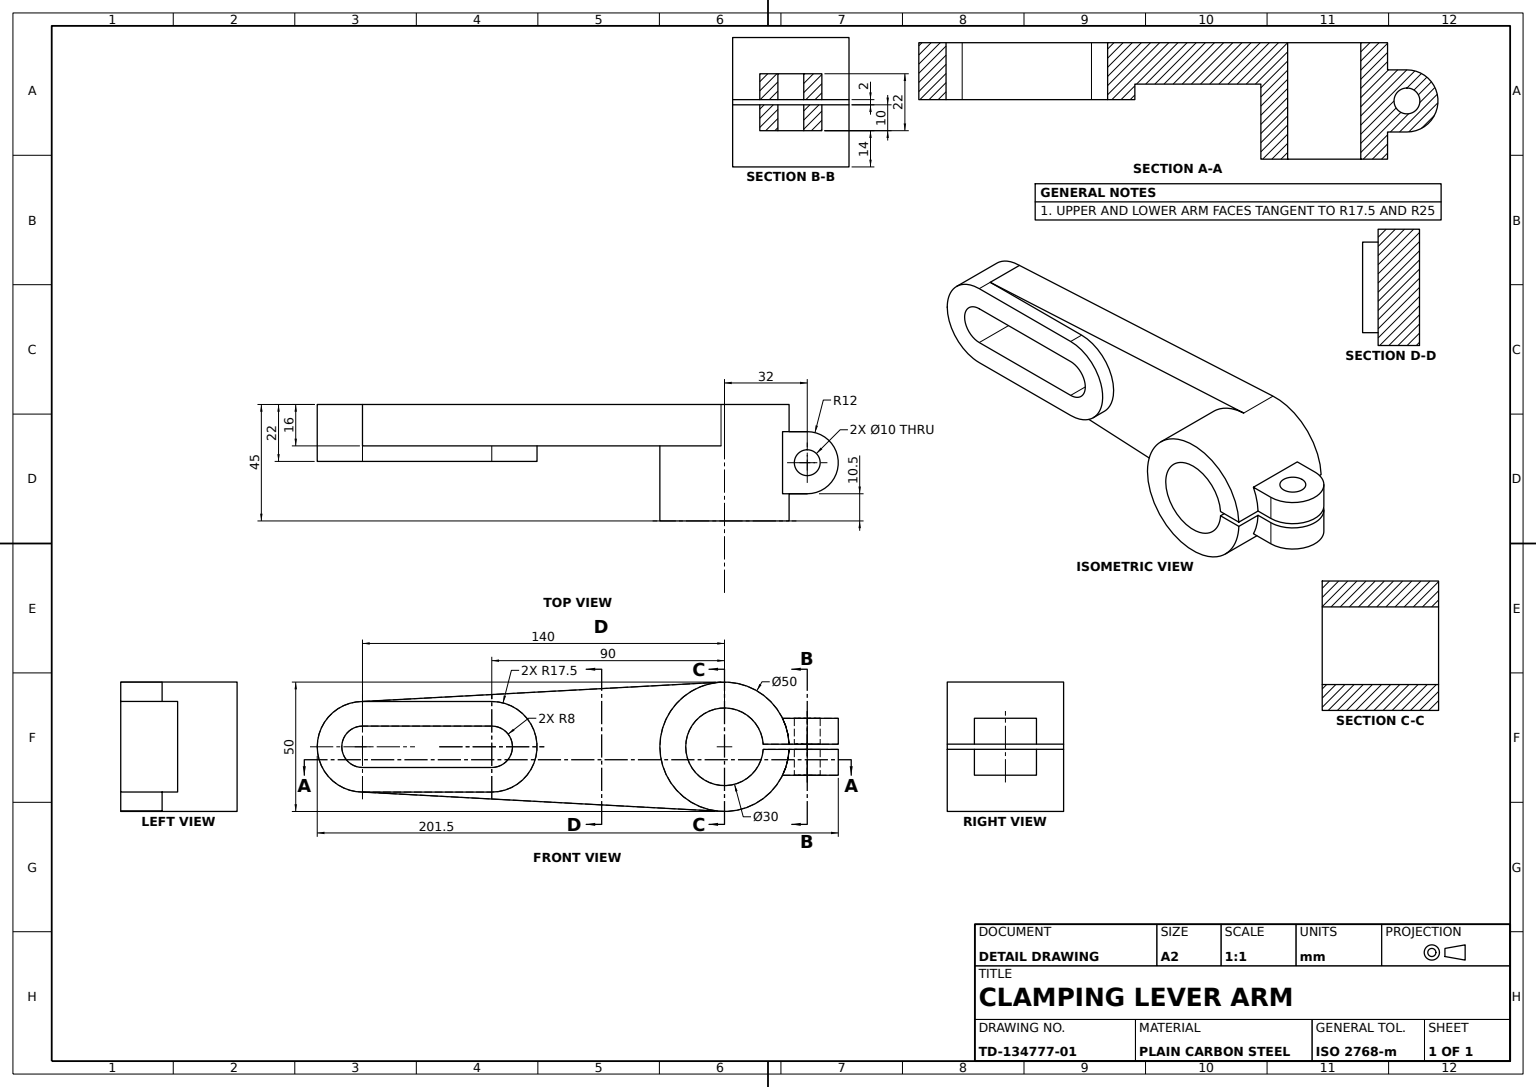
SolidWorks part; units mm, degrees
material "Plain Carbon Steel"
ref_plane "Front Plane" through (0, 0, 0) normal (0, 0, 1) x (1, 0, 0)
ref_plane "Top Plane" through (0, 0, 0) normal (0, 1, 0) x (1, 0, 0)
ref_plane "Right Plane" through (0, 0, 0) normal (1, 0, 0) x (0, 0, -1)
sketch "Hub Profile Sketch" plane through (0, 0, 0) normal (0, 0, 1) x (1, 0, 0)
  circle A0 centre (0, 0) radius 25
  circle A1 centre (0, 0) radius 15
  dimension "D1" = 30
  dimension "D2" = 50
extrude "Shaft Hub Ø50 Bore Ø30" add sketch "Hub Profile Sketch" along normal blind 45
ref_plane "Arm Sketch Plane" through (0, 0, 0) normal (0, 0, 1) x (1, 0, 0)
sketch "Slotted End Sketch" plane through (0, 0, 0) normal (0, 0, 1) x (1, 0, 0)
  line L0 (0, 0) -> (-140, 0) construction
  line L1 (-140, 0) -> (-90, 0) construction
  line L2 (-140, 0) -> (-90, 0) construction
  line L3 (-140, 17.5) -> (-90, 17.5)
  line L4 (-140, -17.5) -> (-90, -17.5)
  line L5 (-140, 8) -> (-90, 8)
  line L6 (-140, -8) -> (-90, -8)
  arc A0 (-140, 17.5) -> (-140, -17.5) centre (-140, 0) ccw
  arc A1 (-90, -17.5) -> (-90, 17.5) centre (-90, 0) ccw
  arc A2 (-140, 8) -> (-140, -8) centre (-140, 0) ccw
  arc A3 (-90, -8) -> (-90, 8) centre (-90, 0) ccw
  point P6 (-115, 0)
  point P11 (-115, 0)
  dimension "D1" = 17.5
  dimension "D2" = 8
  dimension "D4" = 90
  dimension "D3" = 140
extrude "Slotted Arm End" add sketch "Slotted End Sketch" along normal blind 22 separate body
sketch "Arm Web Sketch" plane through (0, 0, 0) normal (0, 0, 1) x (1, 0, 0)
  line L0 (-140, 17.5) -> (-1.3438, 24.9639)
  line L2 (-140, -17.5) -> (0, -25)
  line L3 (-140, -17.5) -> (-90, -17.5) construction
  line L4 (-140, 17.5) -> (-90, 17.5)
  line L5 (-140, -17.5) -> (-90, -17.5)
  circle A0 centre (0, 0) radius 25 construction
  circle A1 centre (0, 0) radius 25
  arc A2 (-90, 17.5) -> (-90, -17.5) centre (-90, 0) cw
extrude "Arm Web" add sketch "Arm Web Sketch" along normal blind 16 contours L4 A2 L5 L2 A1 L0
ref_plane "Clamp Lug Sketch Plane" through (0, 0, 0) normal (0, 1, 0) x (1, 0, 0)
sketch "Clamp Lug Sketch" plane through (0, 0, 0) normal (0, 1, 0) x (1, 0, 0)
  line L0 (32, -34.5) -> (25, -34.5)
  line L1 (25, -45) -> (25, 0) construction
  line L3 (25, -10.5) -> (32, -10.5)
  line L7 (25, -34.5) -> (16.6768, -34.5)
  line L8 (16.6768, -34.5) -> (16.6768, -10.5)
  line L9 (16.6768, -10.5) -> (25, -10.5)
  arc A0 (32, -34.5) -> (32, -10.5) centre (32, -22.5) ccw
  circle A1 centre (32, -22.5) radius 5
  dimension "D1" = 22.5
  dimension "D3" = 10
  dimension "D4" = 12
  dimension "D2" = 32
  dimension "D5" = 8.3232
extrude "Clamp Lug" add sketch "Clamp Lug Sketch" along normal mid plane 22
sketch "Clamp Slit Sketch" plane through (0, 0, 45) normal (0, 0, 1) x (1, 0, 0)
  line L0 (15, 0) -> (43.9637, 0) construction
  line L1 (14.9666, -1) -> (44, -1)
  line L2 (14.9666, 1) -> (43.9273, 1)
  line L4 (44, -11) -> (44, 11) construction
  line L5 (43.9273, 1) -> (47.1313, 1)
  line L6 (0, 1) -> (60.8828, 1) construction
  line L7 (0, -1) -> (60.8828, -1) construction
  line L8 (0, 0) -> (60.8828, 0) construction
  line L9 (47.1313, 1) -> (47.1313, -1)
  line L10 (47.1313, -1) -> (44, -1)
  arc A0 (14.9666, -1) -> (14.9666, 1) centre (0, 0) ccw
  circle A1 centre (0, 0) radius 25 construction
  dimension "D3" = 15
  dimension "D1" = 1
  dimension "D4" = 43.9273
  dimension "D5" = 47.1313
  dimension "D2" = 1
extrude "Clamp Slit 1mm" cut sketch "Clamp Slit Sketch" against normal through all
